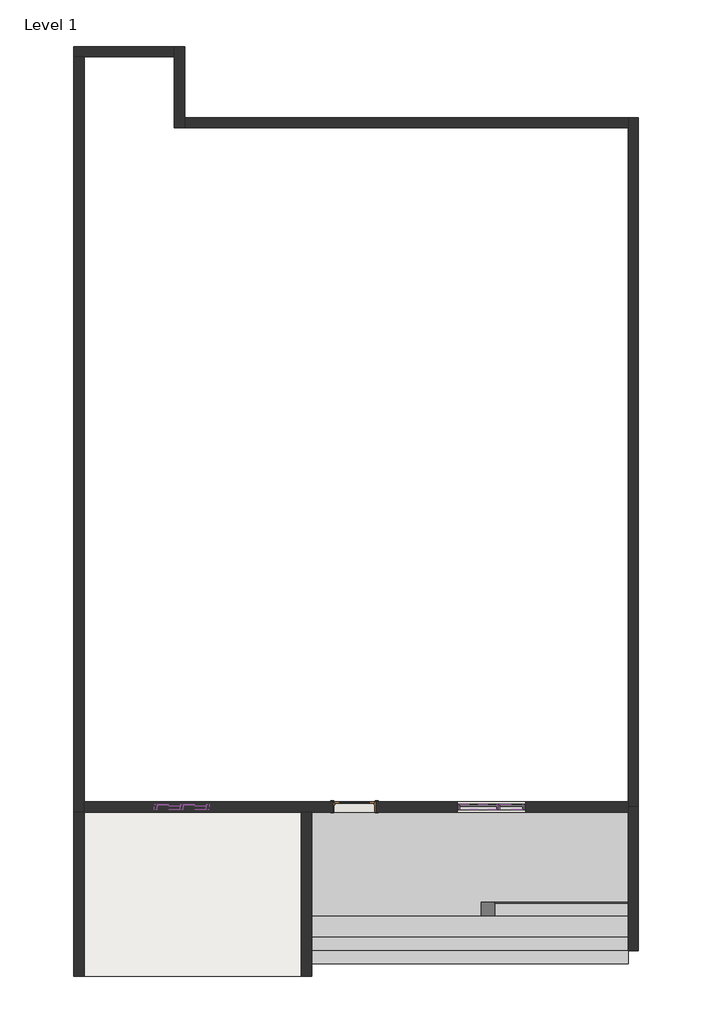
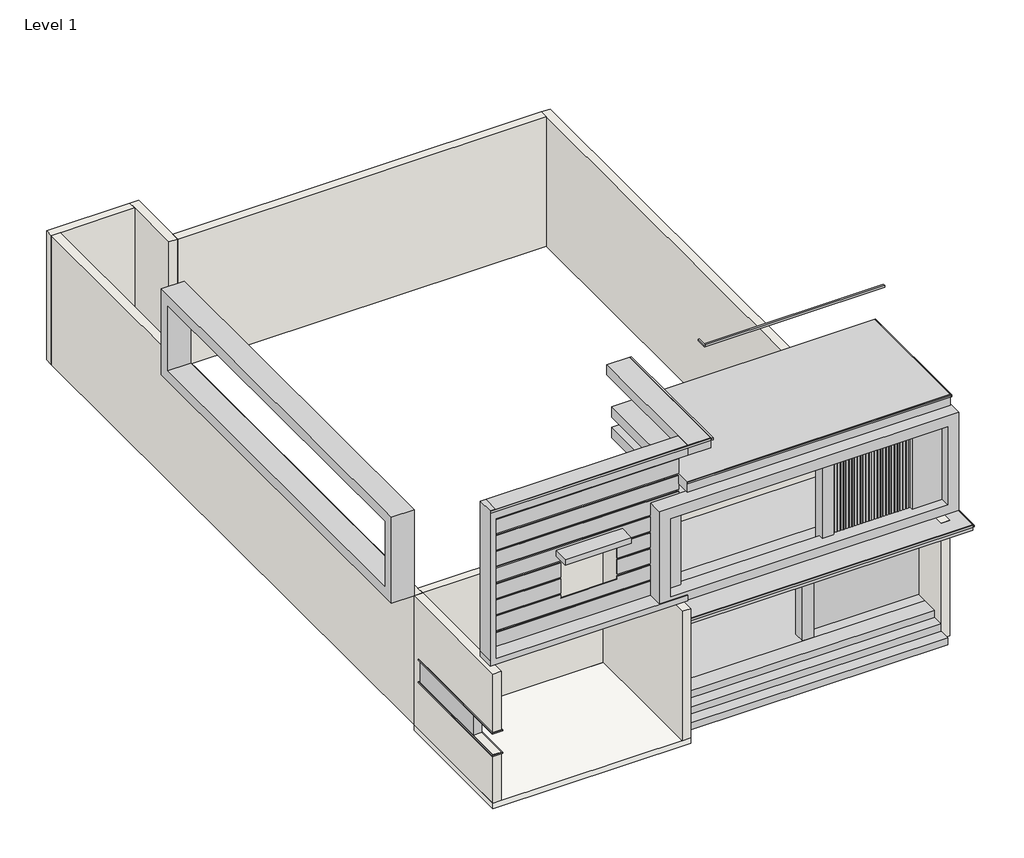
# One storey: 14 members, 9 walls, 4 plates, 1 door, 1 proxy, 1 slab.
"""IFC4 building model written with IfcOpenShell, lengths in millimetres."""

from ifc_helpers import new_model, si_unit, frame, origin, origin_with_axes, place, context, project, spatial, polyline, outline, extrude, faceted_brep, transform, mapped, element, save
from components import generic_models_1_generic_models_1_72e2fdcd, door_868ee8a9, member_0b7646a3, member_c1df12fd, member_fedd83b6, member_c17f1be2, member_d73967ec, member_bdc0ab2a, system_panel_glazed_57bc90b1, system_panel_glazed_0557794d, system_panel_glazed_5c6be660

model = new_model("IFC4")

# Units and contexts
model_context = context("Model", 3, world=origin())
ifc_project = project(units=[si_unit("LENGTHUNIT", "METRE", prefix="MILLI")], contexts=[model_context])

# Site, building, storey
site = spatial("IfcSite", under=ifc_project)
building = spatial("IfcBuilding", under=site)
storey = spatial("IfcBuildingStorey", under=building, Name="Level 1", Elevation=0.0)

# Proxy
placement = place(None, origin())
generic_models_1_generic_models_1_shape = generic_models_1_generic_models_1_72e2fdcd(model_context)
element("IfcBuildingElementProxy", 1, Name="Generic Models 1 : Generic Models 1", ObjectType="Generic Models 1 : Generic Models 1", at=placement, inside=storey, context=model_context, shape_type="MappedRepresentation", body=[
    mapped(generic_models_1_generic_models_1_shape, transform((0.0, 0.0, 0.0), x_axis=(1.0, 0.0, 0.0), y_axis=(0.0, 1.0, 0.0), z_axis=(0.0, 0.0, 1.0))),
])

# Door
door_shape = door_868ee8a9(model_context)
element("IfcDoor", 2, ObjectType="Door-Interior-Single-1_Panel-Wood : 36\" x 84\"", at=placement, inside=storey, context=model_context, shape_type="MappedRepresentation", body=[
    mapped(door_shape, transform((-4295.7909398, -2780.5898025, 609.6), x_axis=(-1.0, 0.0, 0.0), y_axis=(0.0, -1.0, 0.0), z_axis=(0.0, 0.0, 1.0))),
])

# Members
member_shape = member_0b7646a3(model_context)
element("IfcMember", 3, ObjectType="Rectangular Mullion : 2.5\" x 5\" rectangular", at=placement, inside=storey, context=model_context, shape_type="MappedRepresentation", body=[
    mapped(member_shape, transform((-7597.7909398, -2783.7648025, 2768.6), x_axis=(0.0, 0.0, 1.0), y_axis=(0.0, -1.0, 0.0), z_axis=(1.0, 0.0, 0.0))),
])
element("IfcMember", 4, ObjectType="Rectangular Mullion : 2.5\" x 5\" rectangular", at=placement, inside=storey, context=model_context, shape_type="MappedRepresentation", body=[
    mapped(member_shape, transform((-8175.6409398, -2783.7648025, 2768.6), x_axis=(0.0, 0.0, 1.0), y_axis=(0.0, -1.0, 0.0), z_axis=(1.0, 0.0, 0.0))),
])
element("IfcMember", 5, ObjectType="Rectangular Mullion : 2.5\" x 5\" rectangular", at=placement, inside=storey, context=model_context, shape_type="MappedRepresentation", body=[
    mapped(member_shape, transform((-549.2909398, -2783.7648025, 2768.6), x_axis=(0.0, 0.0, 1.0), y_axis=(0.0, -1.0, 0.0), z_axis=(1.0, 0.0, 0.0))),
])
element("IfcMember", 6, ObjectType="Rectangular Mullion : 2.5\" x 5\" rectangular", at=placement, inside=storey, context=model_context, shape_type="MappedRepresentation", body=[
    mapped(member_shape, transform((-8689.9909398, -2783.7648025, 1219.2), x_axis=(0.0, 0.0, -1.0), y_axis=(0.0, -1.0, 0.0), z_axis=(-1.0, 0.0, 0.0))),
])
element("IfcMember", 7, ObjectType="Rectangular Mullion : 2.5\" x 5\" rectangular", at=placement, inside=storey, context=model_context, shape_type="MappedRepresentation", body=[
    mapped(member_shape, transform((-8112.1409398, -2783.7648025, 1219.2), x_axis=(0.0, 0.0, -1.0), y_axis=(0.0, -1.0, 0.0), z_axis=(-1.0, 0.0, 0.0))),
])
element("IfcMember", 8, ObjectType="Rectangular Mullion : 2.5\" x 5\" rectangular", at=placement, inside=storey, context=model_context, shape_type="MappedRepresentation", body=[
    mapped(member_shape, transform((-1063.6409398, -2783.7648025, 914.4), x_axis=(0.0, 0.0, -1.0), y_axis=(0.0, -1.0, 0.0), z_axis=(-1.0, 0.0, 0.0))),
])
member_2_shape = member_c1df12fd(model_context)
element("IfcMember", 9, ObjectType="Rectangular Mullion : 2.5\" x 5\" rectangular", at=placement, inside=storey, context=model_context, shape_type="MappedRepresentation", body=[
    mapped(member_2_shape, transform((-8143.8909398, -2783.7648025, 1219.2), x_axis=(1.0, 0.0, 0.0), y_axis=(0.0, -1.0, 0.0), z_axis=(0.0, 0.0, -1.0))),
])
member_3_shape = member_fedd83b6(model_context)
element("IfcMember", 10, ObjectType="Rectangular Mullion : 2.5\" x 5\" rectangular", at=placement, inside=storey, context=model_context, shape_type="MappedRepresentation", body=[
    mapped(member_3_shape, transform((-8753.4909398, -2783.7648025, 2768.6), x_axis=(-1.0, 0.0, 0.0), y_axis=(0.0, -1.0, 0.0), z_axis=(0.0, 0.0, 1.0))),
])
element("IfcMember", 11, ObjectType="Rectangular Mullion : 2.5\" x 5\" rectangular", at=placement, inside=storey, context=model_context, shape_type="MappedRepresentation", body=[
    mapped(member_3_shape, transform((-7534.2909398, -2783.7648025, 1219.2), x_axis=(1.0, 0.0, 0.0), y_axis=(0.0, -1.0, 0.0), z_axis=(0.0, 0.0, -1.0))),
])
member_4_shape = member_c17f1be2(model_context)
element("IfcMember", 12, ObjectType="Rectangular Mullion : 2.5\" x 5\" rectangular", at=placement, inside=storey, context=model_context, shape_type="MappedRepresentation", body=[
    mapped(member_4_shape, transform((-1946.2909398, -2783.7648025, 914.4), x_axis=(0.0, 0.0, -1.0), y_axis=(0.0, -1.0, 0.0), z_axis=(-1.0, 0.0, 0.0))),
])
member_5_shape = member_d73967ec(model_context)
element("IfcMember", 13, ObjectType="Rectangular Mullion : 2.5\" x 5\" rectangular", at=placement, inside=storey, context=model_context, shape_type="MappedRepresentation", body=[
    mapped(member_5_shape, transform((-1095.3909398, -2783.7648025, 914.4), x_axis=(1.0, 0.0, 0.0), y_axis=(0.0, -1.0, 0.0), z_axis=(0.0, 0.0, -1.0))),
])
element("IfcMember", 14, ObjectType="Rectangular Mullion : 2.5\" x 5\" rectangular", at=placement, inside=storey, context=model_context, shape_type="MappedRepresentation", body=[
    mapped(member_4_shape, transform((-1127.1409398, -2783.7648025, 2768.6), x_axis=(0.0, 0.0, 1.0), y_axis=(0.0, -1.0, 0.0), z_axis=(1.0, 0.0, 0.0))),
])
member_6_shape = member_bdc0ab2a(model_context)
element("IfcMember", 15, ObjectType="Rectangular Mullion : 2.5\" x 5\" rectangular", at=placement, inside=storey, context=model_context, shape_type="MappedRepresentation", body=[
    mapped(member_6_shape, transform((-2009.7909398, -2783.7648025, 2768.6), x_axis=(-1.0, 0.0, 0.0), y_axis=(0.0, -1.0, 0.0), z_axis=(0.0, 0.0, 1.0))),
])
element("IfcMember", 16, ObjectType="Rectangular Mullion : 2.5\" x 5\" rectangular", at=placement, inside=storey, context=model_context, shape_type="MappedRepresentation", body=[
    mapped(member_6_shape, transform((-485.7909398, -2783.7648025, 914.4), x_axis=(1.0, 0.0, 0.0), y_axis=(0.0, -1.0, 0.0), z_axis=(0.0, 0.0, -1.0))),
])

# Plates
system_panel_glazed_shape = system_panel_glazed_57bc90b1(model_context)
element("IfcPlate", 17, ObjectType="System Panel : Glazed", at=placement, inside=storey, context=model_context, shape_type="MappedRepresentation", body=[
    mapped(system_panel_glazed_shape, transform((-8432.8159398, -2783.7648025, 1282.7), x_axis=(1.0, 0.0, 0.0), y_axis=(0.0, 1.0, 0.0), z_axis=(0.0, 0.0, 1.0))),
])
element("IfcPlate", 18, ObjectType="System Panel : Glazed", at=placement, inside=storey, context=model_context, shape_type="MappedRepresentation", body=[
    mapped(system_panel_glazed_shape, transform((-7854.9659398, -2783.7648025, 1282.7), x_axis=(1.0, 0.0, 0.0), y_axis=(0.0, 1.0, 0.0), z_axis=(0.0, 0.0, 1.0))),
])
system_panel_glazed_2_shape = system_panel_glazed_0557794d(model_context)
element("IfcPlate", 19, ObjectType="System Panel : Glazed", at=placement, inside=storey, context=model_context, shape_type="MappedRepresentation", body=[
    mapped(system_panel_glazed_2_shape, transform((-1536.7159398, -2783.7648025, 977.9), x_axis=(1.0, 0.0, 0.0), y_axis=(0.0, 1.0, 0.0), z_axis=(0.0, 0.0, 1.0))),
])
system_panel_glazed_3_shape = system_panel_glazed_5c6be660(model_context)
element("IfcPlate", 20, ObjectType="System Panel : Glazed", at=placement, inside=storey, context=model_context, shape_type="MappedRepresentation", body=[
    mapped(system_panel_glazed_3_shape, transform((-806.4659398, -2783.7648025, 977.9), x_axis=(1.0, 0.0, 0.0), y_axis=(0.0, 1.0, 0.0), z_axis=(0.0, 0.0, 1.0))),
])

# Slab
element("IfcSlab", 21, ObjectType="6\"", at=placement, inside=storey, context=model_context, shape_type="SweptSolid", body=[
    extrude(outline(polyline([(-5248.2909398, -2898.0648025), (-5248.2909398, -6555.6648025), (-10544.1909398, -6555.6648025), (-10544.1909398, -2898.0648025), (-5248.2909398, -2898.0648025)])), frame((0.0, 0.0, -152.4), z_axis=(0.0, 0.0, 1.0), x_axis=(1.0, 0.0, 0.0)), (0.0, 0.0, 1.0), 152.4),
])

# Walls
element("IfcWall", 22, ObjectType="9\" wall", at=placement, inside=storey, context=model_context, shape_type="Brep", body=[
    faceted_brep([(-10315.5909398, -2898.0648025, 0.0), (-10315.5909398, -2669.4648025, 0.0), (-10315.5909398, 13923.3493277, 0.0), (-10315.5909398, 13923.3493277, 3657.6), (-10315.5909398, -2669.4648025, 3657.6), (-10315.5909398, -2898.0648025, 3657.6), (-10544.1909398, -2898.0648025, 0.0), (-10544.1909398, -2898.0648025, 3657.6), (-10544.1909398, 13923.3493277, 3657.6), (-10544.1909398, 13923.3493277, 0.0)], [[[0, 1, 2, 3, 4, 5]], [[6, 7, 8, 9]], [[2, 1, 0, 6, 9]], [[5, 4, 3, 8, 7]], [[0, 5, 7, 6]], [[3, 2, 9, 8]]]),
])
element("IfcWall", 23, ObjectType="9\" wall", at=placement, inside=storey, context=model_context, shape_type="Brep", body=[
    faceted_brep([(1800.2090602, -2669.4648025, 0.0), (-10315.5909398, -2669.4648025, 0.0), (-10315.5909398, -2669.4648025, 3657.6), (1800.2090602, -2669.4648025, 3657.6), (-4778.3909398, -2669.4648025, 2768.6), (-4778.3909398, -2669.4648025, 609.6), (-3813.1909398, -2669.4648025, 609.6), (-3813.1909398, -2669.4648025, 2768.6), (-8753.4909398, -2669.4648025, 2768.6), (-8753.4909398, -2669.4648025, 1219.2), (-7534.2909398, -2669.4648025, 1219.2), (-7534.2909398, -2669.4648025, 2768.6), (-2009.7909398, -2669.4648025, 2768.6), (-2009.7909398, -2669.4648025, 914.4), (-485.7909398, -2669.4648025, 914.4), (-485.7909398, -2669.4648025, 2768.6), (-10315.5909398, -2898.0648025, 0.0), (-5476.8909398, -2898.0648025, 0.0), (-5248.2909398, -2898.0648025, 0.0), (1800.2090602, -2898.0648025, 0.0), (1800.2090602, -2898.0648025, 3260.1762568), (1800.2090602, -2898.0648025, 3657.6), (-5248.2909398, -2898.0648025, 3657.6), (-5476.8909398, -2898.0648025, 3657.6), (-10315.5909398, -2898.0648025, 3657.6), (-4778.3909398, -2898.0648025, 609.6), (-4778.3909398, -2898.0648025, 2768.6), (-3813.1909398, -2898.0648025, 2768.6), (-3813.1909398, -2898.0648025, 609.6), (-8753.4909398, -2898.0648025, 1219.2), (-8753.4909398, -2898.0648025, 2768.6), (-7534.2909398, -2898.0648025, 2768.6), (-7534.2909398, -2898.0648025, 1219.2), (-2009.7909398, -2898.0648025, 914.4), (-2009.7909398, -2898.0648025, 2768.6), (-485.7909398, -2898.0648025, 2768.6), (-485.7909398, -2898.0648025, 914.4), (1800.2090602, -2783.7648025, 0.0)], [[[0, 1, 2, 3], [4, 5, 6, 7], [8, 9, 10, 11], [12, 13, 14, 15]], [[16, 17, 18, 19, 20, 21, 22, 23, 24], [25, 26, 27, 28], [29, 30, 31, 32], [33, 34, 35, 36]], [[1, 0, 37, 19, 18, 17, 16]], [[3, 2, 24, 23, 22, 21]], [[2, 1, 16, 24]], [[19, 37, 0, 3, 21, 20]], [[25, 5, 4, 26]], [[26, 4, 7, 27]], [[27, 7, 6, 28]], [[5, 25, 28, 6]], [[29, 9, 8, 30]], [[30, 8, 11, 31]], [[10, 32, 31, 11]], [[9, 29, 32, 10]], [[33, 13, 12, 34]], [[34, 12, 15, 35]], [[14, 36, 35, 15]], [[13, 33, 36, 14]]]),
])
element("IfcWall", 24, ObjectType="9\" wall", at=placement, inside=storey, context=model_context, shape_type="Brep", body=[
    faceted_brep([(1800.2090602, 12570.5351975, 0.0), (1800.2090602, 12341.9351975, 0.0), (1800.2090602, -2669.4648025, 0.0), (1800.2090602, -2783.7648025, 0.0), (1800.2090602, -2783.7648025, 3260.1762568), (1800.2090602, -2898.0648025, 3260.1762568), (1800.2090602, -2898.0648025, 3657.6), (1800.2090602, -2669.4648025, 3657.6), (1800.2090602, 12341.9351975, 3657.6), (1800.2090602, 12570.5351975, 3657.6), (2028.8090602, 12570.5351975, 0.0), (2028.8090602, 12570.5351975, 3657.6), (2028.8090602, -2898.0648025, 3657.6), (2028.8090602, -2898.0648025, 3260.1762568), (2028.8090602, -2783.7648025, 3260.1762568), (2028.8090602, -2783.7648025, 0.0)], [[[0, 1, 2, 3, 4, 5, 6, 7, 8, 9]], [[10, 11, 12, 13, 14, 15]], [[3, 2, 1, 0, 10, 15]], [[9, 8, 7, 6, 12, 11]], [[0, 9, 11, 10]], [[4, 3, 15, 14]], [[13, 5, 4, 14]], [[6, 5, 13, 12]]]),
])
element("IfcWall", 25, ObjectType="9\" wall", at=placement, inside=storey, context=model_context, shape_type="Brep", body=[
    faceted_brep([(-8309.5689749, 14151.9493277, 0.0), (-8309.5689749, 13923.3493277, 0.0), (-8309.5689749, 12341.9351975, 0.0), (-8309.5689749, 12341.9351975, 3657.6), (-8309.5689749, 13923.3493277, 3657.6), (-8309.5689749, 14151.9493277, 3657.6), (-8080.9689749, 14151.9493277, 0.0), (-8080.9689749, 14151.9493277, 3657.6), (-8080.9689749, 12570.5351975, 3657.6), (-8080.9689749, 12341.9351975, 3657.6), (-8080.9689749, 12341.9351975, 0.0), (-8080.9689749, 12570.5351975, 0.0)], [[[0, 1, 2, 3, 4, 5]], [[6, 7, 8, 9, 10, 11]], [[2, 1, 0, 6, 11, 10]], [[5, 4, 3, 9, 8, 7]], [[0, 5, 7, 6]], [[3, 2, 10, 9]]]),
])
element("IfcWall", 26, ObjectType="9\" wall", at=placement, inside=storey, context=model_context, shape_type="Brep", body=[
    faceted_brep([(-10544.1909398, 13923.3493277, 0.0), (-10315.5909398, 13923.3493277, 0.0), (-8309.5689749, 13923.3493277, 0.0), (-8309.5689749, 13923.3493277, 3657.6), (-10315.5909398, 13923.3493277, 3657.6), (-10544.1909398, 13923.3493277, 3657.6), (-10544.1909398, 14151.9493277, 0.0), (-10544.1909398, 14151.9493277, 3657.6), (-8309.5689749, 14151.9493277, 3657.6), (-8309.5689749, 14151.9493277, 0.0)], [[[0, 1, 2, 3, 4, 5]], [[6, 7, 8, 9]], [[2, 1, 0, 6, 9]], [[5, 4, 3, 8, 7]], [[3, 2, 9, 8]], [[0, 5, 7, 6]]]),
])
element("IfcWall", 27, ObjectType="9\" wall", at=placement, inside=storey, context=model_context, shape_type="SweptSolid", body=[
    extrude(outline(polyline([(1800.2090602, 12341.9351975), (-8080.9689749, 12341.9351975), (-8080.9689749, 12570.5351975), (1800.2090602, 12570.5351975), (1800.2090602, 12341.9351975)])), origin_with_axes(), (0.0, 0.0, 1.0), 3657.6),
])
element("IfcWall", 28, ObjectType="9\" wall", at=placement, inside=storey, context=model_context, shape_type="SweptSolid", body=[
    extrude(outline(polyline([(-2898.0648025, 0.0), (-6555.6648025, 0.0), (-6555.6648025, 1371.6), (-3155.6170173, 1371.6), (-3155.6170173, 1981.2), (-6555.6648025, 1981.2), (-6555.6648025, 3657.6), (-2898.0648025, 3657.6), (-2898.0648025, 0.0)])), frame((-10544.1909398, 0.0, 0.0), z_axis=(1.0, 0.0, 0.0), x_axis=(0.0, 1.0, 0.0)), (0.0, 0.0, 1.0), 228.6),
])
element("IfcWall", 29, ObjectType="9\" wall", at=placement, inside=storey, context=model_context, shape_type="SweptSolid", body=[
    extrude(outline(polyline([(-5476.8909398, -6555.6648025), (-5476.8909398, -2898.0648025), (-5248.2909398, -2898.0648025), (-5248.2909398, -6555.6648025), (-5476.8909398, -6555.6648025)])), origin_with_axes(), (0.0, 0.0, 1.0), 3657.6),
])
element("IfcWall", 30, ObjectType="9\" wall", at=placement, inside=storey, context=model_context, shape_type="Brep", body=[
    faceted_brep([(1800.2090602, -2783.7648025, 0.0), (1800.2090602, -2898.0648025, 0.0), (1800.2090602, -5984.1648025, 0.0), (1800.2090602, -5984.1648025, 3260.1762568), (1800.2090602, -2898.0648025, 3260.1762568), (1800.2090602, -2783.7648025, 3260.1762568), (2028.8090602, -2783.7648025, 0.0), (2028.8090602, -2783.7648025, 3260.1762568), (2028.8090602, -2898.0648025, 3260.1762568), (2028.8090602, -5984.1648025, 3260.1762568), (2028.8090602, -5984.1648025, 0.0)], [[[0, 1, 2, 3, 4, 5]], [[6, 7, 8, 9, 10]], [[2, 1, 0, 6, 10]], [[3, 2, 10, 9]], [[5, 4, 3, 9, 8, 7]], [[0, 5, 7, 6]]]),
])

save(model, "model.ifc")

# Revit data of these elements
# Type "Door-Interior-Single-1_Panel-Wood : 36\" x 84\""
#   Type Mark = "8"
#   Assembly Code = "C1020300"
#   Analytic Construction = "Wooden"
#   Top Rail = 0' - 4 11/16"
#   Thickness = 0' - 1 3/8"
#   Thermal Resistance (R) = 2.5876 (h·ft²·°F)/BTU
#   Swing Angle [instance default] = 90.00°
#   Stiles = 0' - 4 3/4"
#   Rough Width = 3' - 2"
#   Rough Height = 7' - 1"
#   Height = 7' - 0"
#   Width = 3' - 0"
#   Heat Transfer Coefficient (U) = 0.3865 BTU/(h·ft²·°F)
#   Bottom Rail = 0' - 9 1/8"
#   Trim Material = Cherry
#   Panel Material = Cherry
#   Frame Material = Cherry
#   Door Handle Material = Aluminum
#   Visual Light Transmittance = 0
#   Solar Heat Gain Coefficient = 0
#   Wall Closure = (empty or 0)
#   Function = (empty or 0)
# Type "Rectangular Mullion : 2.5\" x 5\" rectangular"
#   built-in parameter 1007304 = 0.416667 (stored number, unit not read)
#   built-in parameter 1007301 = 0.104167 (stored number, unit not read)
#   built-in parameter 1007300 = 0.104167 (stored number, unit not read)
# Type "System Panel : Glazed"
#   Construction Type Id = "GSP4R"
#   Analytic Construction = "1/8 in Pilkington single glazing"
#   Visual Light Transmittance = 0.9
#   Solar Heat Gain Coefficient = 0.86
#   Heat Transfer Coefficient (U) = 1.18115 BTU/(h·ft²·°F)
#   Define Thermal Properties by = 1
# Type "6\""
#   Assembly Code = "B1010"
#   Function = 0
#   Layers, outside or top first: 0' - 6" no material (function 1)
# Type "9\" wall"
#   Assembly Code = "B2010"
#   Layers, outside or top first: 0' - 9" "Laminate, Ivory, Matte" (function 1)
# Element 1 (IfcBuildingElementProxy, "Generic Models 1 : Generic Models 1")
#   Phase Created = New Construction
#   Materials on its faces: "wood", "Laminate, Ivory, Matte", "window wall", "balcony extrusion", "Gypsum Wall Board", "tile"
# Element 2 (IfcDoor, "Door-Interior-Single-1_Panel-Wood : 36\" x 84\"")
#   Swing Angle = 90.00°
#   Phase Created = New Construction
#   Materials on its faces: "Cherry", "Aluminum"
# Elements 3, 4, 5, 6, 7, 8, 9, 10, 11, 12, 13, 14, 15, 16 (IfcMember, "Rectangular Mullion : 2.5\" x 5\" rectangular")
#   Phase Created = New Construction
# Elements 17, 18, 19, 20 (IfcPlate, "System Panel : Glazed")
#   Phase Created = New Construction
#   Materials on its faces: "Glass"
# Element 21 (IfcSlab, "6\"")
#   Height Offset From Level = 0' - 0"
#   Phase Created = New Construction
#   Materials on its faces: "Default Floor"
# Elements 22, 23, 24, 25, 26, 27, 28, 29 (IfcWall, "9\" wall")
#   Top Offset = 0' - 0"
#   Base Offset = 0' - 0"
#   wall height = 12' - 0"
#   Phase Created = New Construction
#   Base Constraint = Level 1
#   Top Constraint = Level 2
#   Materials on its faces: "Laminate, Ivory, Matte"
# Element 30 (IfcWall, "9\" wall")
#   Top Offset = -1' - 3.6466"
#   Base Offset = 0' - 0"
#   wall height = 10' - 8.3534"
#   Phase Created = New Construction
#   Base Constraint = Level 1
#   Top Constraint = Level 2
#   Materials on its faces: "Laminate, Ivory, Matte"
# Materials
#   "Cherry": class "Wood", colour RGB 226 177 128, transparency 0, Description = "Prunus Serotina", Cost = 0
#   "Aluminum": class "Metal", colour RGB 247 247 247, transparency 0, Description = "Aluminum 6061", Cost = 0
#   "Laminate, Ivory, Matte": class "Plastic", colour RGB 247 247 239, transparency 0, Description = "Plastic Laminate - Ivory, Matte", Cost = 0
#   "wood": class "Generic", colour RGB 120 120 120, transparency 0, Cost = 0
#   "window wall": class "Generic", colour RGB 120 120 120, transparency 0, Cost = 0
#   "balcony extrusion": class "Generic", colour RGB 120 120 120, transparency 0, Cost = 0
#   "Gypsum Wall Board": class "Generic", colour RGB 127 127 127, transparency 0, Description = "Gypsum Wall Board", Cost = 0
#   "tile": class "Generic", colour RGB 120 120 120, transparency 0, Cost = 0
#   "Glass": class "Glass", colour RGB 0 128 192, transparency 0.75, Description = "Soda Lime Glass", Cost = 0
#   "Default Floor": colour RGB 128 128 128, transparency 0, Cost = 0
